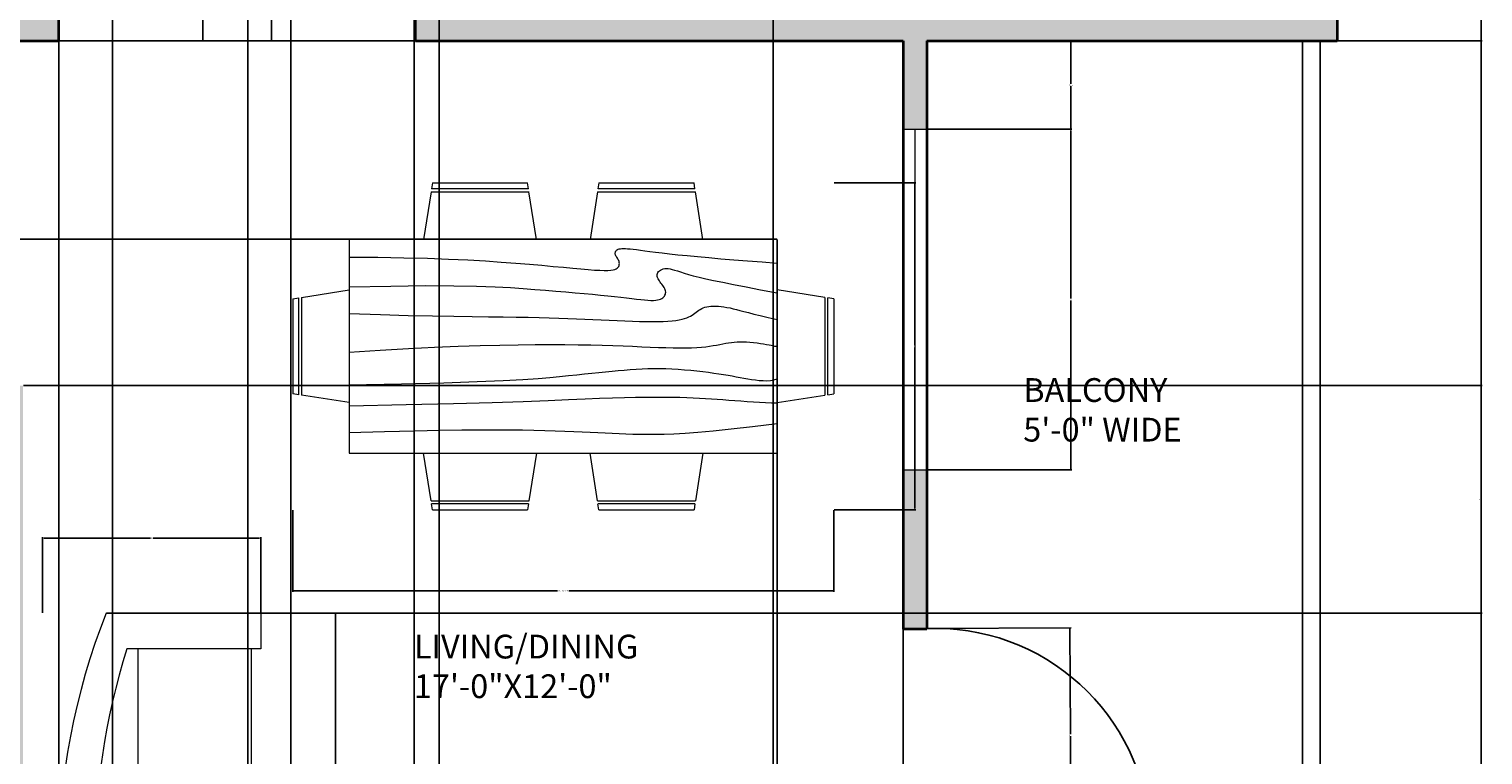
# Model space of a CAD drawing. Units: inches. Extents: x -29 to 443, y -589 to 39.
# Tile 4 of 5: x 139 to 384, y -275 to -153. Entities that reach past the tile are written whole.
import ezdxf

# ---------------------------------------------------------------- set-up
doc = ezdxf.new("R2010")
doc.units = ezdxf.units.IN
for name, color, linetype, lineweight in [('A-ANNO-DIMS', 2, 'Continuous', 18), ('A-AREA-IDEN', 7, 'Continuous', 18), ('A-DOOR', 3, 'Continuous', 25), ('A-FLOR-HRAL', 8, 'Continuous', 25), ('A-FURN', 9, 'Continuous', 18), ('A-GLAZ', 4, 'Continuous', 18), ('A-WALL', 7, 'Continuous', 35)]:
    doc.layers.add(name, color=color, linetype=linetype, lineweight=lineweight)
doc.layers.add('A-WALL-PATT', color=251, linetype='Continuous', lineweight=13, true_color=0x636466)
doc.styles.get("Standard").update_dxf_attribs({"font": 'arial.ttf'})
doc.dimstyles.get("Standard").update_dxf_attribs({"dimtxt": 0.18, "dimasz": 0.18, "dimexe": 0.18, "dimexo": 0.0625, "dimgap": 0.09, "dimtad": 0, "dimtih": 1, "dimtoh": 1, "dimdec": 4, "dimzin": 0, "dimdsep": 46, "dimtxsty": 'Standard', "dimcen": 0.09, "dimadec": 0, "dimazin": 0, "dimtfac": 1, "dimtdec": 4, "dimtofl": 0, "dimtmove": 0, "dimatfit": 3, "dimfxl": 1, "dimtolj": 1, "dimtzin": 0, "dimarcsym": 0})

# ---------------------------------------------------------------- blocks, each defined once
blk = doc.blocks.new('*U3')
for p, q in [((0, 0), (0, -6)), ((40, 0), (40, -6))]:
    blk.add_line(p, q)
blk.add_lwpolyline([(0, 0), (0, 40), (1.75, 40), (1.75, 0)], close=True)
blk.add_arc((0, 0), 40, 0, 90)
blk = doc.blocks.new('Sofa - Roundback 7 ft.')
for p, q in [((-12.00002, -32.4421), (-12.00003, -6.5971)), ((11.99997, -32.4421), (11.99998, -6.5971)), ((-36.000027, -34), (-36.000027, -11.4696)), ((35.99998, -34), (35.99998, -11.4696)), ((-35.999844, -13.3819), (35.9998, -13.3819)), ((-36.000027, -32.4421), (35.99998, -32.4421))]:
    blk.add_line(p, q)
for points in [[(-36.000027, -34), (-42.000027, -34), (-42.000027, -8)], [(41.99998, -8), (41.99998, -34), (35.99998, -34)]]:
    blk.add_lwpolyline(points)
for centre, radius, start, end in [((0, -114.25), 114.25, 68.43141, 111.5686), ((-0.00001, -127.1968), 121.1968, 72.72033, 107.2797)]:
    blk.add_arc(centre, radius, start, end)
blk = doc.blocks.new('Dining Set - 36 x 72 in.')
for p, q in [((-22, 27.5), (-22.1562, 26.50042)), ((-22, 27.5), (-6, 27.5)), ((-5.8437, 26.49966), (-6, 27.5)), ((6, 27.5), (5.8438, 26.50042)), ((6, 27.5), (22, 27.5)), ((22.1563, 26.49966), (22, 27.5)), ((-22.2343, 26.00059), (-23.4847, 17.99762)), ((-22.2304, 26), (-5.7608, 26)), ((-5.8416, 26.5), (-22.1534, 26.5)), ((-4.5152, 17.99762), (-5.7655, 25.99926)), ((5.7657, 26.00059), (4.5153, 17.99762)), ((5.7696, 26), (22.2392, 26)), ((22.1584, 26.5), (5.8466, 26.5)), ((23.4848, 17.99762), (22.2345, 25.99926)), ((36, 18), (-36, 18)), ((-36, 18), (-36, -18)), ((36, -18), (36, 18)), ((-45.5, 8), (-44.5004, 8.15617)), ((-45.5, 8), (-45.5, -8)), ((-44.5, -8.15843), (-44.5, 8.15338)), ((-44.0006, 8.23428), (-35.9976, 9.48474)), ((-44, 8.23041), (-44, -8.23915)), ((44.0006, 8.23428), (35.9976, 9.48474)), ((44, 8.23041), (44, -8.23915)), ((44.5, -8.15843), (44.5, 8.15338)), ((45.5, 8), (44.5005, 8.15617)), ((45.5, 8), (45.5, -8)), ((-44.4997, -8.15631), (-45.5, -8)), ((-35.9976, -9.48476), (-43.9993, -8.2345)), ((35.9976, -9.48476), (43.9993, -8.2345)), ((44.4997, -8.15631), (45.5, -8)), ((-36, -18), (36, -18)), ((-22.2343, -26.0006), (-23.4847, -17.99762)), ((-4.5152, -17.99762), (-5.7655, -25.99928)), ((5.7657, -26.0006), (4.5153, -17.99762)), ((23.4848, -17.99762), (22.2345, -25.99928)), ((-22.2304, -26), (-5.7608, -26)), ((-22, -27.5), (-22.1562, -26.50044)), ((-5.8416, -26.5), (-22.1534, -26.5)), ((-5.8437, -26.49967), (-6, -27.5)), ((5.7696, -26), (22.2392, -26)), ((6, -27.5), (5.8438, -26.50044)), ((22.1584, -26.5), (5.8466, -26.5)), ((22.1563, -26.49967), (22, -27.5)), ((-22, -27.5), (-6, -27.5)), ((6, -27.5), (22, -27.5))]:
    blk.add_line(p, q)
for points in [[(-36, 15), (-31.1772, 14.97754), (-26.8079, 14.91406), (-22.8538, 14.81543), (-19.276, 14.6875), (-16.0362, 14.53613), (-13.0957, 14.36718), (-10.4159, 14.18652), (-7.9583, 14), (-5.6904, 13.81315), (-3.6035, 13.63021), (-1.6954, 13.45508), (0.0365, 13.29166), (1.5945, 13.14388), (2.9811, 13.01562), (4.1988, 12.9108), (5.25, 12.83333), (6.1393, 12.78613), (6.8802, 12.76823), (7.4883, 12.77767), (7.9792, 12.8125), (8.3685, 12.87077), (8.6719, 12.95052), (8.9049, 13.0498), (9.0833, 13.16666), (9.2205, 13.29899), (9.3216, 13.44401), (9.3895, 13.59879), (9.4271, 13.76041), (9.4373, 13.92594), (9.4232, 14.09245), (9.3875, 14.257), (9.3333, 14.41666), (9.2638, 14.56917), (9.1836, 14.71484), (9.0975, 14.85465), (9.0104, 14.98958), (8.9272, 15.1206), (8.8529, 15.2487), (8.7922, 15.37483), (8.75, 15.5), (8.7305, 15.62467), (8.7344, 15.74739), (8.7617, 15.86621), (8.8125, 15.97916), (8.8867, 16.08431), (8.9844, 16.17968), (9.1055, 16.26334), (9.25, 16.33333), (9.4189, 16.38802), (9.6172, 16.42708), (9.8506, 16.45052), (10.125, 16.45833), (10.4463, 16.45052), (10.8203, 16.42708), (11.2529, 16.38802), (11.75, 16.33333), (12.3184, 16.26318), (12.9694, 16.17838), (13.7151, 16.07991), (14.5677, 15.96875), (15.5395, 15.84586), (16.6426, 15.71224), (17.8893, 15.56884), (19.2917, 15.41666), (20.859, 15.25667), (22.5879, 15.08984), (24.4721, 14.91715), (26.5052, 14.73958), (28.6809, 14.5581), (30.9929, 14.3737), (33.4347, 14.18733), (36, 14)], [(-36, 10), (-28.9766, 10.14274), (-23.1725, 10.20442), (-18.4241, 10.19775), (-14.5677, 10.13541), (-11.4399, 10.03011), (-8.877, 9.89453), (-6.7154, 9.74137), (-4.7917, 9.58333), (-2.9698, 9.43082), (-1.2246, 9.28515), (0.4415, 9.14534), (2.026, 9.01041), (3.5266, 8.87939), (4.9408, 8.7513), (6.266, 8.62516), (7.5, 8.5), (8.6411, 8.37549), (9.6914, 8.2539), (10.6538, 8.13818), (11.5312, 8.03125), (12.3267, 7.93603), (13.043, 7.85547), (13.6831, 7.79248), (14.25, 7.75), (14.7471, 7.7303), (15.1797, 7.73307), (15.5537, 7.75732), (15.875, 7.80208), (16.1494, 7.86637), (16.3828, 7.94922), (16.5811, 8.04964), (16.75, 8.16666), (16.8944, 8.29915), (17.0143, 8.44531), (17.1089, 8.60319), (17.1771, 8.77083), (17.218, 8.94629), (17.2305, 9.1276), (17.2137, 9.31282), (17.1667, 9.5), (17.0895, 9.6875), (16.987, 9.875), (16.8649, 10.0625), (16.7292, 10.25), (16.5856, 10.4375), (16.4401, 10.625), (16.2985, 10.8125), (16.1667, 11), (16.05, 11.18733), (15.9518, 11.3737), (15.8752, 11.5581), (15.8229, 11.73958), (15.798, 11.91715), (15.8034, 12.08984), (15.842, 12.25667), (15.9167, 12.41666), (16.0295, 12.56836), (16.1784, 12.70833), (16.3605, 12.83268), (16.5729, 12.9375), (16.8127, 13.01888), (17.0768, 13.07291), (17.3625, 13.0957), (17.6667, 13.08333), (17.9894, 13.03312), (18.3418, 12.94726), (18.7382, 12.82918), (19.1927, 12.68229), (19.7195, 12.51001), (20.3327, 12.31575), (21.0465, 12.10294), (21.875, 11.875), (22.8357, 11.63354), (23.959, 11.37304), (25.2786, 11.08618), (26.8282, 10.76562), (28.6414, 10.40405), (30.752, 9.99414), (33.1936, 9.52856), (36, 9)], [(-36, 5.5), (-30.7157, 5.3348), (-26.069, 5.20963), (-21.9946, 5.11767), (-18.4271, 5.05208), (-15.3009, 5.00602), (-12.5508, 4.97265), (-10.1112, 4.94515), (-7.9167, 4.91666), (-5.909, 4.88167), (-4.0586, 4.83984), (-2.3429, 4.79215), (-0.7396, 4.73958), (0.7739, 4.6831), (2.22, 4.6237), (3.6213, 4.56233), (5, 4.5), (6.373, 4.43782), (7.7344, 4.3776), (9.0723, 4.32129), (10.375, 4.27083), (11.6309, 4.22819), (12.8281, 4.19531), (13.9551, 4.17415), (15, 4.16666), (15.954, 4.17448), (16.819, 4.19791), (17.6001, 4.23698), (18.3021, 4.29166), (18.9299, 4.36198), (19.4883, 4.44791), (19.9823, 4.54948), (20.4167, 4.66666), (20.7969, 4.79899), (21.1302, 4.94401), (21.4245, 5.09879), (21.6875, 5.26041), (21.9271, 5.42594), (22.1511, 5.59245), (22.3672, 5.757), (22.5834, 5.91666), (22.8065, 6.06868), (23.0404, 6.21093), (23.2879, 6.34147), (23.5521, 6.45833), (23.8358, 6.55957), (24.142, 6.64323), (24.4735, 6.70735), (24.8334, 6.75), (25.2235, 6.76969), (25.642, 6.76692), (26.0858, 6.74267), (26.5521, 6.69791), (27.0379, 6.63362), (27.5404, 6.55078), (28.0565, 6.45036), (28.5834, 6.33333), (29.1242, 6.19987), (29.7071, 6.04687), (30.3661, 5.87044), (31.1354, 5.66666), (32.0493, 5.43164), (33.142, 5.16146), (34.4475, 4.85221), (36, 4.5)], [(-36, -1), (-30.7915, -0.6591), (-26.0195, -0.38216), (-21.6519, -0.16284), (-17.6563, 0.00521), (-14.0005, 0.12833), (-10.6523, 0.21289), (-7.5796, 0.26522), (-4.75, 0.29166), (-2.134, 0.29793), (0.2878, 0.28711), (2.5317, 0.26163), (4.6146, 0.22396), (6.5529, 0.17651), (8.3633, 0.12174), (10.0623, 0.06209), (11.6667, 0), (13.1899, -0.06201), (14.6341, -0.1211), (15.9982, -0.17432), (17.2813, -0.21875), (18.4823, -0.25147), (19.6003, -0.26953), (20.6343, -0.27002), (21.5834, -0.25), (22.4481, -0.20768), (23.2357, -0.14584), (23.9549, -0.06836), (24.6146, 0.02083), (25.2235, 0.11784), (25.7904, 0.21875), (26.3241, 0.31966), (26.8334, 0.41666), (27.3265, 0.50618), (27.8099, 0.58593), (28.2894, 0.65397), (28.7709, 0.70833), (29.2601, 0.74707), (29.763, 0.76823), (30.2855, 0.76985), (30.8334, 0.75), (31.4088, 0.70784), (31.9994, 0.64713), (32.589, 0.57275), (33.1615, 0.48958), (33.7008, 0.4025), (34.1908, 0.3164), (34.6153, 0.23616), (34.9584, 0.16666), (35.2099, 0.11165), (35.3848, 0.07031), (35.504, 0.04069), (35.5886, 0.02083), (35.6594, 0.00879), (35.7377, 0.0026), (35.8442, 0.00032), (36, 0)], [(-36, -6.5), (-27.1843, -6.31267), (-20.084, -6.1263), (-14.469, -5.9419), (-10.1094, -5.76042), (-6.7752, -5.58285), (-4.2363, -5.41016), (-2.2629, -5.24333), (-0.625, -5.08334), (0.8708, -4.93099), (2.2715, -4.78646), (3.5872, -4.64974), (4.8281, -4.52084), (6.0046, -4.39974), (7.127, -4.28646), (8.2053, -4.18099), (9.25, -4.08334), (10.2705, -3.99382), (11.2734, -3.91407), (12.2647, -3.84603), (13.25, -3.79167), (14.2354, -3.75293), (15.2266, -3.73177), (16.2295, -3.73015), (17.25, -3.75), (18.2912, -3.79248), (19.3451, -3.85547), (20.4009, -3.93604), (21.4479, -4.03125), (22.4754, -4.13819), (23.4727, -4.25391), (24.4289, -4.37549), (25.3334, -4.5), (26.1785, -4.62492), (26.9694, -4.74935), (27.7145, -4.87281), (28.4219, -4.99479), (29.1, -5.11483), (29.7572, -5.23242), (30.4016, -5.34709), (31.0417, -5.45834), (31.6837, -5.56437), (32.3262, -5.65821), (32.9658, -5.73153), (33.599, -5.77604), (34.2224, -5.78345), (34.8327, -5.74545), (35.4264, -5.65373), (36, -5.5)], [(-36, -10), (-26.4022, -9.81299), (-18.4675, -9.62891), (-11.9839, -9.45069), (-6.7396, -9.28125), (-2.5226, -9.12354), (0.8789, -8.98047), (3.6769, -8.85498), (6.0833, -8.75), (8.2767, -8.66765), (10.3021, -8.60677), (12.1712, -8.56543), (13.8958, -8.54167), (15.4876, -8.53353), (16.9583, -8.53907), (18.3197, -8.55632), (19.5834, -8.58334), (20.7616, -8.61841), (21.8685, -8.66081), (22.9188, -8.71004), (23.9271, -8.76563), (24.9081, -8.82707), (25.8763, -8.89388), (26.8465, -8.96558), (27.8334, -9.04167), (28.8474, -9.12118), (29.8828, -9.20117), (30.93, -9.27824), (31.9792, -9.34896), (33.0205, -9.40991), (34.0443, -9.45768), (35.0407, -9.48885), (36, -9.5)], [(-36, -14.5), (-30.0881, -14.33513), (-25.0332, -14.21224), (-20.7312, -14.12647), (-17.0781, -14.07292), (-13.97, -14.04671), (-11.3027, -14.04297), (-8.9724, -14.05681), (-6.875, -14.08334), (-4.9224, -14.11833), (-3.0905, -14.16016), (-1.3709, -14.20785), (0.2448, -14.26042), (1.7647, -14.3169), (3.1973, -14.3763), (4.5507, -14.43767), (5.8333, -14.5), (7.0554, -14.5621), (8.235, -14.62175), (9.3922, -14.67652), (10.5469, -14.72396), (11.7192, -14.76164), (12.929, -14.78711), (14.1965, -14.79794), (15.5417, -14.79167), (16.9933, -14.76424), (18.6152, -14.70508), (20.4804, -14.60197), (22.6615, -14.44271), (25.2312, -14.21509), (28.2624, -13.9069), (31.8277, -13.50594), (36, -13)]]:
    blk.add_lwpolyline(points)
blk = doc.blocks.new('*D30')
at = {"layer": 'A-ANNO-DIMS', "color": 0, "lineweight": -2, "transparency": 16777216}
for p, q in [((178.45, -250.92), (191.17, -250.92)), ((190.99, -251.1), (190.99, -292.74)), ((190.99, -334.74), (190.99, -293.11)), ((178.45, -334.92), (191.17, -334.92))]:
    blk.add_line(p, q, dxfattribs=at)
at = {"layer": 'A-ANNO-DIMS', "color": 0, "transparency": 16777216}
for points in [[(190.96, -251.1), (191.02, -251.1), (190.99, -250.92)], [(190.96, -334.74), (191.02, -334.74), (190.99, -334.92)]]:
    blk.add_solid(points, dxfattribs=at)
at = {"layer": 'Defpoints', "color": 0, "transparency": 16777216}
for p in [(178.39, -250.92), (190.99, -250.92), (178.39, -334.92)]:
    blk.add_point(p, dxfattribs=at)
at = {"layer": 'A-ANNO-DIMS', "color": 0, "transparency": 16777216, "insert": (190.99, -292.92), "char_height": 0.18, "attachment_point": 5}
blk.add_mtext('\\A1;SOFA 84', dxfattribs=at)
blk = doc.blocks.new('*D31')
at = {"layer": 'A-ANNO-DIMS', "color": 0, "lineweight": -2, "transparency": 16777216}
for p, q in [((141.72, -250.86), (141.72, -238.14)), ((141.9, -238.32), (159.84, -238.32)), ((178.21, -238.32), (160.28, -238.32)), ((178.39, -250.86), (178.39, -238.14))]:
    blk.add_line(p, q, dxfattribs=at)
at = {"layer": 'A-ANNO-DIMS', "color": 0, "transparency": 16777216}
for points in [[(141.9, -238.29), (141.9, -238.35), (141.72, -238.32)], [(178.21, -238.29), (178.21, -238.35), (178.39, -238.32)]]:
    blk.add_solid(points, dxfattribs=at)
at = {"layer": 'Defpoints', "color": 0, "transparency": 16777216}
for p in [(141.72, -238.32), (141.72, -250.92), (178.39, -250.92)]:
    blk.add_point(p, dxfattribs=at)
at = {"layer": 'A-ANNO-DIMS', "color": 0, "transparency": 16777216, "insert": (160.06, -238.32), "char_height": 0.18, "attachment_point": 5}
blk.add_mtext('\\A1;37', dxfattribs=at)
blk = doc.blocks.new('*D32')
at = {"layer": 'A-ANNO-DIMS', "color": 0, "lineweight": -2, "transparency": 16777216}
for p, q in [((183.78, -233.57), (183.78, -247.33)), ((274.78, -233.57), (274.78, -247.33)), ((183.96, -247.15), (228.33, -247.15)), ((274.6, -247.15), (230.24, -247.15))]:
    blk.add_line(p, q, dxfattribs=at)
at = {"layer": 'A-ANNO-DIMS', "color": 0, "transparency": 16777216}
for points in [[(183.96, -247.12), (183.96, -247.18), (183.78, -247.15)], [(274.6, -247.12), (274.6, -247.18), (274.78, -247.15)]]:
    blk.add_solid(points, dxfattribs=at)
at = {"layer": 'Defpoints', "color": 0, "transparency": 16777216}
for p in [(183.78, -233.5), (274.78, -233.5), (274.78, -247.15)]:
    blk.add_point(p, dxfattribs=at)
at = {"layer": 'A-ANNO-DIMS', "color": 0, "transparency": 16777216, "insert": (229.28, -247.15), "char_height": 0.18, "attachment_point": 5}
blk.add_mtext('\\A1;DINING SET 91', dxfattribs=at)
blk = doc.blocks.new('*D33')
at = {"layer": 'A-ANNO-DIMS', "color": 0, "lineweight": -2, "transparency": 16777216}
for p, q in [((274.85, -178.5), (288.61, -178.5)), ((288.43, -178.68), (288.43, -205.82)), ((288.43, -233.32), (288.43, -206.18)), ((274.85, -233.5), (288.61, -233.5))]:
    blk.add_line(p, q, dxfattribs=at)
at = {"layer": 'A-ANNO-DIMS', "color": 0, "transparency": 16777216}
for points in [[(288.4, -178.68), (288.46, -178.68), (288.43, -178.5)], [(288.4, -233.32), (288.46, -233.32), (288.43, -233.5)]]:
    blk.add_solid(points, dxfattribs=at)
at = {"layer": 'Defpoints', "color": 0, "transparency": 16777216}
for p in [(274.78, -178.5), (288.43, -178.5), (274.78, -233.5)]:
    blk.add_point(p, dxfattribs=at)
at = {"layer": 'A-ANNO-DIMS', "color": 0, "transparency": 16777216, "insert": (288.43, -206), "char_height": 0.18, "attachment_point": 5}
blk.add_mtext('\\A1;55', dxfattribs=at)
blk = doc.blocks.new('*D40')
at = {"layer": 'A-ANNO-DIMS', "color": 0, "lineweight": -2, "transparency": 16777216}
for p, q in [((208.44, 5.32), (208.44, -492.89)), ((264.58, 5.32), (264.58, -492.89)), ((208.62, -492.71), (236.11, -492.71)), ((264.4, -492.71), (236.9, -492.71))]:
    blk.add_line(p, q, dxfattribs=at)
at = {"layer": 'A-ANNO-DIMS', "color": 0, "transparency": 16777216}
for points in [[(208.62, -492.68), (208.62, -492.74), (208.44, -492.71)], [(264.4, -492.68), (264.4, -492.74), (264.58, -492.71)]]:
    blk.add_solid(points, dxfattribs=at)
at = {"layer": 'Defpoints', "color": 0, "transparency": 16777216}
for p in [(208.44, 5.39), (264.58, 5.39), (208.44, -492.71)]:
    blk.add_point(p, dxfattribs=at)
at = {"layer": 'A-ANNO-DIMS', "color": 0, "transparency": 16777216, "insert": (236.51, -492.71), "char_height": 0.18, "attachment_point": 5}
blk.add_mtext('\\A1;56.14', dxfattribs=at)
blk = doc.blocks.new('*D44')
at = {"layer": 'A-ANNO-DIMS', "color": 0, "lineweight": -2, "transparency": 16777216}
for p, q in [((359.5, 14.39), (383.85, 14.39)), ((383.67, 14.21), (383.67, -69.93)), ((383.67, -154.43), (383.67, -70.3)), ((359.5, -154.61), (383.85, -154.61))]:
    blk.add_line(p, q, dxfattribs=at)
at = {"layer": 'A-ANNO-DIMS', "color": 0, "transparency": 16777216}
for points in [[(383.64, 14.21), (383.7, 14.21), (383.67, 14.39)], [(383.64, -154.43), (383.7, -154.43), (383.67, -154.61)]]:
    blk.add_solid(points, dxfattribs=at)
at = {"layer": 'Defpoints', "color": 0, "transparency": 16777216}
for p in [(359.44, 14.39), (359.44, -154.61), (383.67, -154.61)]:
    blk.add_point(p, dxfattribs=at)
at = {"layer": 'A-ANNO-DIMS', "color": 0, "transparency": 16777216, "insert": (383.67, -70.11), "char_height": 0.18, "attachment_point": 5}
blk.add_mtext('\\A1;169', dxfattribs=at)
blk = doc.blocks.new('*D45')
at = {"layer": 'A-ANNO-DIMS', "color": 0, "lineweight": -2, "transparency": 16777216}
for p, q in [((359.5, -154.61), (383.85, -154.61)), ((383.67, -154.79), (383.67, -226.43)), ((383.67, -298.43), (383.67, -226.8)), ((359.5, -298.61), (383.85, -298.61))]:
    blk.add_line(p, q, dxfattribs=at)
at = {"layer": 'A-ANNO-DIMS', "color": 0, "transparency": 16777216}
for points in [[(383.64, -154.79), (383.7, -154.79), (383.67, -154.61)], [(383.64, -298.43), (383.7, -298.43), (383.67, -298.61)]]:
    blk.add_solid(points, dxfattribs=at)
at = {"layer": 'Defpoints', "color": 0, "transparency": 16777216}
for p in [(359.44, -154.61), (359.44, -298.61), (383.67, -298.61)]:
    blk.add_point(p, dxfattribs=at)
at = {"layer": 'A-ANNO-DIMS', "color": 0, "transparency": 16777216, "insert": (383.67, -226.61), "char_height": 0.18, "attachment_point": 5}
blk.add_mtext('\\A1;144', dxfattribs=at)
blk = doc.blocks.new('*D51')
at = {"layer": 'A-ANNO-DIMS', "color": 0, "lineweight": -2, "transparency": 16777216}
for p, q in [((144.5, -141.61), (168.85, -141.61)), ((168.67, -141.79), (168.67, -147.93)), ((168.67, -154.43), (168.67, -148.3)), ((144.5, -154.61), (168.85, -154.61))]:
    blk.add_line(p, q, dxfattribs=at)
at = {"layer": 'A-ANNO-DIMS', "color": 0, "transparency": 16777216}
for points in [[(168.64, -141.79), (168.7, -141.79), (168.67, -141.61)], [(168.64, -154.43), (168.7, -154.43), (168.67, -154.61)]]:
    blk.add_solid(points, dxfattribs=at)
at = {"layer": 'Defpoints', "color": 0, "transparency": 16777216}
for p in [(144.44, -141.61), (144.44, -154.61), (168.67, -154.61)]:
    blk.add_point(p, dxfattribs=at)
at = {"layer": 'A-ANNO-DIMS', "color": 0, "transparency": 16777216, "insert": (168.67, -148.11), "char_height": 0.18, "attachment_point": 5}
blk.add_mtext('\\A1;13', dxfattribs=at)
blk = doc.blocks.new('*D52')
at = {"layer": 'A-ANNO-DIMS', "color": 0, "lineweight": -2, "transparency": 16777216}
for p, q in [((153.44, -94.68), (153.44, -492.89)), ((183.44, -94.68), (183.44, -492.89)), ((153.62, -492.71), (168.22, -492.71)), ((183.26, -492.71), (168.65, -492.71))]:
    blk.add_line(p, q, dxfattribs=at)
at = {"layer": 'A-ANNO-DIMS', "color": 0, "transparency": 16777216}
for points in [[(153.62, -492.68), (153.62, -492.74), (153.44, -492.71)], [(183.26, -492.68), (183.26, -492.74), (183.44, -492.71)]]:
    blk.add_solid(points, dxfattribs=at)
at = {"layer": 'Defpoints', "color": 0, "transparency": 16777216}
for p in [(153.44, -94.61), (183.44, -94.61), (183.44, -492.71)]:
    blk.add_point(p, dxfattribs=at)
at = {"layer": 'A-ANNO-DIMS', "color": 0, "transparency": 16777216, "insert": (168.44, -492.71), "char_height": 0.18, "attachment_point": 5}
blk.add_mtext('\\A1;30', dxfattribs=at)
blk = doc.blocks.new('*D55')
at = {"layer": 'A-ANNO-DIMS', "color": 0, "lineweight": -2, "transparency": 16777216}
for p, q in [((290.34, -253.47), (314.69, -253.36)), ((314.51, -253.54), (314.59, -271.25)), ((314.66, -289.33), (314.59, -271.62)), ((290.5, -289.61), (314.85, -289.51))]:
    blk.add_line(p, q, dxfattribs=at)
at = {"layer": 'A-ANNO-DIMS', "color": 0, "transparency": 16777216}
for points in [[(314.54, -253.54), (314.48, -253.54), (314.51, -253.36)], [(314.69, -289.33), (314.63, -289.33), (314.67, -289.51)]]:
    blk.add_solid(points, dxfattribs=at)
at = {"layer": 'Defpoints', "color": 0, "transparency": 16777216}
for p in [(290.28, -253.47), (290.44, -289.61), (314.67, -289.51)]:
    blk.add_point(p, dxfattribs=at)
at = {"layer": 'A-ANNO-DIMS', "color": 0, "transparency": 16777216, "insert": (314.59, -271.44), "char_height": 0.18, "attachment_point": 5}
blk.add_mtext('\\A1;36.15', dxfattribs=at)
blk = doc.blocks.new('*D63')
at = {"layer": 'A-ANNO-DIMS', "color": 0, "lineweight": -2, "transparency": 16777216}
for p, q in [((204.37, -144.61), (180.03, -144.61)), ((180.21, -144.79), (180.21, -149.43)), ((180.21, -154.43), (180.21, -149.8)), ((204.37, -154.61), (180.03, -154.61))]:
    blk.add_line(p, q, dxfattribs=at)
at = {"layer": 'A-ANNO-DIMS', "color": 0, "transparency": 16777216}
for points in [[(180.18, -144.79), (180.24, -144.79), (180.21, -144.61)], [(180.18, -154.43), (180.24, -154.43), (180.21, -154.61)]]:
    blk.add_solid(points, dxfattribs=at)
at = {"layer": 'Defpoints', "color": 0, "transparency": 16777216}
for p in [(180.21, -144.61), (204.44, -144.61), (204.44, -154.61)]:
    blk.add_point(p, dxfattribs=at)
at = {"layer": 'A-ANNO-DIMS', "color": 0, "transparency": 16777216, "insert": (180.21, -149.61), "char_height": 0.18, "attachment_point": 5}
blk.add_mtext('\\A1;10', dxfattribs=at)
blk = doc.blocks.new('*D68')
at = {"layer": 'A-ANNO-DIMS', "color": 0, "lineweight": -2, "transparency": 16777216}
for p, q in [((176.21, -22.71), (176.21, -492.89)), ((204.21, -33.21), (204.21, -492.89)), ((176.39, -492.71), (189.99, -492.71)), ((204.03, -492.71), (190.43, -492.71))]:
    blk.add_line(p, q, dxfattribs=at)
at = {"layer": 'A-ANNO-DIMS', "color": 0, "transparency": 16777216}
for points in [[(176.39, -492.68), (176.39, -492.74), (176.21, -492.71)], [(204.03, -492.68), (204.03, -492.74), (204.21, -492.71)]]:
    blk.add_solid(points, dxfattribs=at)
at = {"layer": 'Defpoints', "color": 0, "transparency": 16777216}
for p in [(176.21, -22.65), (204.21, -33.15), (204.21, -492.71)]:
    blk.add_point(p, dxfattribs=at)
at = {"layer": 'A-ANNO-DIMS', "color": 0, "transparency": 16777216, "insert": (190.21, -492.71), "char_height": 0.18, "attachment_point": 5}
blk.add_mtext('\\A1;28', dxfattribs=at)
blk = doc.blocks.new('*D71')
at = {"layer": 'A-ANNO-DIMS', "color": 0, "lineweight": -2, "transparency": 16777216}
for p, q in [((144.44, -94.68), (144.44, -492.89)), ((153.44, -94.68), (153.44, -492.89)), ((144.62, -492.71), (148.79, -492.71)), ((153.26, -492.71), (149.09, -492.71))]:
    blk.add_line(p, q, dxfattribs=at)
at = {"layer": 'A-ANNO-DIMS', "color": 0, "transparency": 16777216}
for points in [[(144.62, -492.68), (144.62, -492.74), (144.44, -492.71)], [(153.26, -492.68), (153.26, -492.74), (153.44, -492.71)]]:
    blk.add_solid(points, dxfattribs=at)
at = {"layer": 'Defpoints', "color": 0, "transparency": 16777216}
for p in [(144.44, -94.61), (153.44, -94.61), (153.44, -492.71)]:
    blk.add_point(p, dxfattribs=at)
at = {"layer": 'A-ANNO-DIMS', "color": 0, "transparency": 16777216, "insert": (148.94, -492.71), "char_height": 0.18, "attachment_point": 5}
blk.add_mtext('\\A1;9', dxfattribs=at)
blk = doc.blocks.new('*D74')
at = {"layer": 'A-ANNO-DIMS', "color": 0, "lineweight": -2, "transparency": 16777216}
for p, q in [((286.44, -169.54), (286.44, -492.89)), ((265.28, -188.07), (265.28, -492.89)), ((265.46, -492.71), (275.46, -492.71)), ((286.26, -492.71), (276.26, -492.71))]:
    blk.add_line(p, q, dxfattribs=at)
at = {"layer": 'A-ANNO-DIMS', "color": 0, "transparency": 16777216}
for points in [[(265.46, -492.68), (265.46, -492.74), (265.28, -492.71)], [(286.26, -492.68), (286.26, -492.74), (286.44, -492.71)]]:
    blk.add_solid(points, dxfattribs=at)
at = {"layer": 'Defpoints', "color": 0, "transparency": 16777216}
for p in [(286.44, -169.48), (265.28, -188), (286.44, -492.71)]:
    blk.add_point(p, dxfattribs=at)
at = {"layer": 'A-ANNO-DIMS', "color": 0, "transparency": 16777216, "insert": (275.86, -492.71), "char_height": 0.18, "attachment_point": 5}
blk.add_mtext('\\A1;21.15', dxfattribs=at)
blk = doc.blocks.new('*D75')
at = {"layer": 'A-ANNO-DIMS', "color": 0, "lineweight": -2, "transparency": 16777216}
for p, q in [((286.37, -154.61), (-28.85, -154.61)), ((-28.67, -154.79), (-28.67, -171.13)), ((-28.67, -187.82), (-28.67, -171.49)), ((265.22, -188), (-28.85, -188))]:
    blk.add_line(p, q, dxfattribs=at)
at = {"layer": 'A-ANNO-DIMS', "color": 0, "transparency": 16777216}
for points in [[(-28.7, -154.79), (-28.64, -154.79), (-28.67, -154.61)], [(-28.7, -187.82), (-28.64, -187.82), (-28.67, -188)]]:
    blk.add_solid(points, dxfattribs=at)
at = {"layer": 'Defpoints', "color": 0, "transparency": 16777216}
for p in [(-28.67, -154.61), (286.44, -154.61), (265.28, -188)]:
    blk.add_point(p, dxfattribs=at)
at = {"layer": 'A-ANNO-DIMS', "color": 0, "transparency": 16777216, "insert": (-28.67, -171.31), "char_height": 0.18, "attachment_point": 5}
blk.add_mtext('\\A1;33.39', dxfattribs=at)
blk = doc.blocks.new('*D77')
at = {"layer": 'A-ANNO-DIMS', "color": 0, "lineweight": -2, "transparency": 16777216}
for p, q in [((290.5, -154.61), (314.85, -154.61)), ((314.67, -154.79), (314.67, -161.86)), ((314.67, -169.3), (314.67, -162.23)), ((290.5, -169.48), (314.85, -169.48))]:
    blk.add_line(p, q, dxfattribs=at)
at = {"layer": 'A-ANNO-DIMS', "color": 0, "transparency": 16777216}
for points in [[(314.64, -154.79), (314.7, -154.79), (314.67, -154.61)], [(314.64, -169.3), (314.7, -169.3), (314.67, -169.48)]]:
    blk.add_solid(points, dxfattribs=at)
at = {"layer": 'Defpoints', "color": 0, "transparency": 16777216}
for p in [(290.44, -154.61), (290.44, -169.48), (314.67, -169.48)]:
    blk.add_point(p, dxfattribs=at)
at = {"layer": 'A-ANNO-DIMS', "color": 0, "transparency": 16777216, "insert": (314.67, -162.05), "char_height": 0.18, "attachment_point": 5}
blk.add_mtext('\\A1;14.863', dxfattribs=at)
blk = doc.blocks.new('*D78')
at = {"layer": 'A-ANNO-DIMS', "color": 0, "lineweight": -2, "transparency": 16777216}
for p, q in [((290.5, -169.48), (314.85, -169.48)), ((314.67, -169.66), (314.67, -197.95)), ((314.67, -226.61), (314.67, -198.32)), ((290.5, -226.79), (314.85, -226.79))]:
    blk.add_line(p, q, dxfattribs=at)
at = {"layer": 'A-ANNO-DIMS', "color": 0, "transparency": 16777216}
for points in [[(314.64, -169.66), (314.7, -169.66), (314.67, -169.48)], [(314.64, -226.61), (314.7, -226.61), (314.67, -226.79)]]:
    blk.add_solid(points, dxfattribs=at)
at = {"layer": 'Defpoints', "color": 0, "transparency": 16777216}
for p in [(290.44, -169.48), (290.44, -226.79), (314.67, -226.79)]:
    blk.add_point(p, dxfattribs=at)
at = {"layer": 'A-ANNO-DIMS', "color": 0, "transparency": 16777216, "insert": (314.67, -198.13), "char_height": 0.18, "attachment_point": 5}
blk.add_mtext('\\A1;57.31', dxfattribs=at)
blk = doc.blocks.new('*D82')
at = {"layer": 'A-ANNO-DIMS', "color": 0, "lineweight": -2, "transparency": 16777216}
for p, q in [((138.5, -212.61), (383.85, -212.61)), ((383.67, -212.79), (383.67, -231.59)), ((383.67, -250.74), (383.67, -231.95)), ((152.45, -250.92), (383.85, -250.92))]:
    blk.add_line(p, q, dxfattribs=at)
at = {"layer": 'A-ANNO-DIMS', "color": 0, "transparency": 16777216}
for points in [[(383.64, -212.79), (383.7, -212.79), (383.67, -212.61)], [(383.64, -250.74), (383.7, -250.74), (383.67, -250.92)]]:
    blk.add_solid(points, dxfattribs=at)
at = {"layer": 'Defpoints', "color": 0, "transparency": 16777216}
for p in [(138.44, -212.61), (152.39, -250.92), (383.67, -250.92)]:
    blk.add_point(p, dxfattribs=at)
at = {"layer": 'A-ANNO-DIMS', "color": 0, "transparency": 16777216, "insert": (383.67, -231.77), "char_height": 0.18, "attachment_point": 5}
blk.add_mtext('\\A1;38.31', dxfattribs=at)

msp = doc.modelspace()

# ---------------------------------------------------------------- hatches: boundary and pattern name
at = {"layer": 'A-WALL-PATT'}
h = msp.add_hatch(color=256, dxfattribs=at)
h.dxf.hatch_style = 1
h.paths.add_polyline_path([(8.4359, 5.3851), (38.6638, 5.3851), (38.6638, 14.3851), (-0.5641, 14.3851), (-0.5641, -161.7206), (8.4359, -161.7206), (8.4359, -154.6149), (98.4359, -154.6149), (98.4359, -169.6149), (102.4359, -169.6149), (102.4359, -154.6149), (144.4359, -154.6149), (144.4359, -141.6149), (140.4359, -141.6149), (140.4359, -150.6149), (8.4359, -150.6149)])
h.paths.add_polyline_path([(153.762, 14.3851), (92.6638, 14.3851), (92.6638, 5.3851), (140.4359, 5.3851), (140.4359, -105.5868), (144.4359, -105.5868), (144.4359, -94.6149), (153.4359, -94.6149), (153.4359, -90.6149), (144.4359, -90.6149), (144.4359, 5.3851), (153.762, 5.3851)])
h.paths.add_polyline_path([(264.576, 14.3851), (189.762, 14.3851), (189.762, 5.3851), (204.4359, 5.3851), (204.4359, -40.0486, -0.11439146), (204.5889, -40.7086), (204.5889, -67.7086, -0.11439146), (204.4359, -68.3685), (204.4359, -90.6149), (183.4359, -90.6149), (183.4359, -94.6149), (204.4359, -94.6149), (204.4359, -108.4622), (208.4359, -108.4622), (208.4359, 5.3851), (264.576, 5.3851)])
h.paths.add_polyline_path([(359.4359, 14.3851), (318.576, 14.3851), (318.576, 5.3851), (350.4359, 5.3851), (350.4359, -150.6149), (208.4359, -150.6149), (208.4359, -144.6149), (204.4359, -144.6149), (204.4359, -154.6149), (286.4359, -154.6149), (286.4359, -169.4775), (290.4359, -169.4775), (290.4359, -154.6149), (359.4359, -154.6149)])
h.paths.add_polyline_path([(8.4359, -212.6149), (98.4359, -212.6149), (102.4359, -212.6149), (102.4359, -199.6149), (98.4359, -199.6149), (98.4359, -208.6149), (8.4359, -208.6149), (8.4359, -197.7206), (-0.5641, -197.7206), (-0.5641, -417.6149), (114.4359, -417.6149), (114.4359, -354.6149), (134.4359, -354.6149), (134.4359, -453.6149), (147.4359, -453.6149), (147.4359, -444.6149), (138.4359, -444.6149), (138.4359, -212.6149), (129.4359, -212.6149), (129.4359, -216.6149), (134.4359, -216.6149), (134.4359, -350.6149), (110.4359, -350.6149), (110.4359, -377.2063, -0.30395766), (111.1497, -378.2719, -0.30395766), (110.4359, -379.3376), (110.4359, -408.6149), (8.4359, -408.6149)])
h.paths.add_polyline_path([(265.0252, -444.6149), (230.4359, -444.6149), (230.4359, -396.6149), (246.223, -396.6149), (246.223, -392.6149), (230.4359, -392.6149), (230.4359, -302.6149), (245.4886, -302.6149), (245.4886, -298.6149), (226.4359, -298.6149), (226.4359, -444.6149), (189.4359, -444.6149), (189.4359, -453.6149), (226.4359, -453.6149), (265.0252, -453.6149)])
h.paths.add_polyline_path([(359.4359, -417.6149), (359.4359, -377.3771), (350.4359, -377.3771), (350.4359, -392.6149), (276.3235, -392.6149), (276.3235, -396.6149), (350.4359, -396.6149), (350.4359, -408.6149), (350.4359, -444.6149), (319.0252, -444.6149), (319.0252, -453.6149), (359.4359, -453.6149)])
h.paths.add_polyline_path([(359.4359, -298.6149), (290.4359, -298.6149), (290.4359, -289.6207), (286.4359, -289.6207), (286.4359, -298.6149), (277.8355, -298.6149), (277.8355, -302.6149), (350.4359, -302.6149), (350.4359, -323.3771), (359.4359, -323.3771)])
h.paths.add_polyline_path([(290.4359, -226.7916), (286.4359, -226.7916), (286.4359, -253.468), (290.4359, -253.468)])

# ---------------------------------------------------------------- linework, layer by layer
at = {"layer": 'A-FLOR-HRAL'}
for p, q in [((353.5994, -154.6149), (353.5994, -298.6149)), ((356.5994, -154.6149), (356.5994, -298.6149))]:
    msp.add_line(p, q, dxfattribs=at)
at = {"layer": 'A-GLAZ'}
for p, q in [((286.4359, -169.4775), (290.4359, -169.4775)), ((288.4359, -169.4775), (288.4359, -226.7916)), ((286.4359, -226.7916), (290.4359, -226.7916))]:
    msp.add_line(p, q, dxfattribs=at)
at = {"layer": 'A-WALL'}
for p, q in [((359.4359, 14.3851), (359.4359, -154.6149)), ((144.4359, -154.6149), (144.4359, -141.6149)), ((204.4359, -154.6149), (204.4359, -144.6149)), ((102.4359, -154.6149), (144.4359, -154.6149)), ((204.4359, -154.6149), (286.4359, -154.6149)), ((286.4359, -154.6149), (286.4359, -253.6149)), ((290.4359, -154.6149), (290.4359, -253.6149)), ((290.4359, -154.6149), (359.4359, -154.6149)), ((290.4359, -253.6149), (286.4359, -253.6149))]:
    msp.add_line(p, q, dxfattribs=at)

# ---------------------------------------------------------------- block references
at = {"layer": 'A-DOOR', "xscale": -0.9038178546105021, "yscale": 0.9038178546105021, "zscale": 0.9038178546105021, "rotation": 270}
msp.add_blockref('*U3', (291.8589, -289.6207), dxfattribs=at)
at = {"layer": 'A-FURN'}
msp.add_blockref('Dining Set - 36 x 72 in.', (229.284, -206.0033), dxfattribs=at)
at = {"layer": 'A-FURN', "rotation": 89.99999967709844}
msp.add_blockref('Sofa - Roundback 7 ft.', (144.3905, -292.9234), dxfattribs=at)

# ---------------------------------------------------------------- texts
at = {"layer": 'A-AREA-IDEN', "char_height": 4, "attachment_point": 1}
for s, width, insert in [('BALCONY\\P5\'-0" WIDE', 32.234328, (306.6588, -211.3646)), ('LIVING/DINING\\P17\'-0"X12\'-0"', 54.511225, (204.1648, -254.5404))]:
    msp.add_mtext_dynamic_manual_height_columns(s, width=width, gutter_width=12.5, heights=[0], dxfattribs=dict(at, insert=insert))

# ---------------------------------------------------------------- dimensions: what is measured, and where the dimension line sits
at = {"layer": 'A-ANNO-DIMS'}
for base, p1, p2, angle, override, picture, middle in [((383.6659, -154.6149), (359.4359, 14.3851), (359.4359, -154.6149), 90, {"dimdec": 0, "dimlfac": 1, "dimrnd": 0, "dimzin": 0, "dimdsep": 46, "dimlunit": 2}, '*D44', (383.6659, -70.1149)), ((168.6659, -154.6149), (144.4359, -141.6149), (144.4359, -154.6149), 270, {"dimdec": 0, "dimlfac": 1, "dimrnd": 0, "dimzin": 0, "dimdsep": 46, "dimlunit": 2}, '*D51', (168.6659, -148.1149)), ((180.2059, -144.6149), (204.4359, -154.6149), (204.4359, -144.6149), 90, {"dimdec": 0, "dimlfac": 1, "dimrnd": 0, "dimzin": 0, "dimdsep": 46, "dimlunit": 2}, '*D63', (180.2059, -149.6149)), ((-28.6698, -154.6149), (265.284, -188.0033), (286.4359, -154.6149), 90, {"dimdec": 2, "dimlfac": 1, "dimrnd": 0, "dimzin": 0, "dimdsep": 46, "dimlunit": 2}, '*D75', (-28.6698, -171.3091)), ((314.6659, -169.4775), (290.4359, -154.6149), (290.4359, -169.4775), 270, {"dimdec": 3, "dimlfac": 1, "dimrnd": 0, "dimzin": 0, "dimdsep": 46, "dimlunit": 2}, '*D77', (314.6659, -162.0462)), ((383.6659, -298.6149), (359.4359, -154.6149), (359.4359, -298.6149), 90, {"dimdec": 0, "dimlfac": 1, "dimrnd": 0, "dimzin": 0, "dimdsep": 46, "dimlunit": 2}, '*D45', (383.6659, -226.6149)), ((314.6659, -226.7916), (290.4359, -169.4775), (290.4359, -226.7916), 270, {"dimdec": 2, "dimlfac": 1, "dimrnd": 0, "dimzin": 0, "dimdsep": 46, "dimlunit": 2}, '*D78', (314.6659, -198.1345)), ((288.434, -178.5033), (274.784, -233.5033), (274.784, -178.5033), 90, {"dimdec": 0, "dimlfac": 1, "dimrnd": 0, "dimzin": 0, "dimdsep": 46, "dimlunit": 2}, '*D33', (288.434, -206.0033)), ((383.6659, -250.9234), (138.4359, -212.6149), (152.3905, -250.9234), 90, {"dimdec": 2, "dimlfac": 1, "dimrnd": 0, "dimzin": 0, "dimdsep": 46, "dimlunit": 2}, '*D82', (383.6659, -231.7692)), ((141.7238, -238.3234), (178.3905, -250.9234), (141.7238, -250.9234), 180, {"dimdec": 0, "dimlfac": 1, "dimrnd": 0, "dimzin": 0, "dimdsep": 46, "dimlunit": 2}, '*D31', (160.0572, -238.3234)), ((314.6657, -289.5085), (290.2772, -253.468), (290.4359, -289.6149), 270.251668, {"dimdec": 2, "dimlfac": 1, "dimrnd": 0, "dimzin": 0, "dimdsep": 46, "dimlunit": 2}, '*D55', (314.5863, -271.435))]:
    dim = msp.add_linear_dim(base=base, p1=p1, p2=p2, angle=angle, dimstyle='Standard', override=override, dxfattribs=at)
    dim.commit()
    dim.dimension.update_dxf_attribs({"geometry": picture, "text_midpoint": middle})
for base, p1, p2, override, picture, middle in [((208.4359, -492.7145), (264.576, 5.3851), (208.4359, 5.3851), {"dimdec": 2, "dimlfac": 1, "dimrnd": 0, "dimzin": 0, "dimdsep": 46, "dimlunit": 2}, '*D40', (236.506, -492.7145)), ((204.211, -492.7145), (176.211, -22.6482), (204.211, -33.1482), {"dimdec": 0, "dimlfac": 1, "dimrnd": 0, "dimzin": 0, "dimdsep": 46, "dimlunit": 2}, '*D68', (190.211, -492.7145)), ((153.4359, -492.7145), (144.4359, -94.6149), (153.4359, -94.6149), {"dimdec": 0, "dimlfac": 1, "dimrnd": 0, "dimzin": 0, "dimdsep": 46, "dimlunit": 2}, '*D71', (148.9359, -492.7145)), ((183.4359, -492.7145), (153.4359, -94.6149), (183.4359, -94.6149), {"dimdec": 0, "dimlfac": 1, "dimrnd": 0, "dimzin": 0, "dimdsep": 46, "dimlunit": 2}, '*D52', (168.4359, -492.7145)), ((286.4359, -492.7145), (265.284, -188.0033), (286.4359, -169.4775), {"dimdec": 2, "dimlfac": 1, "dimrnd": 0, "dimzin": 0, "dimdsep": 46, "dimlunit": 2}, '*D74', (275.86, -492.7145))]:
    dim = msp.add_linear_dim(base=base, p1=p1, p2=p2, dimstyle='Standard', override=override, dxfattribs=at)
    dim.commit()
    dim.dimension.update_dxf_attribs({"geometry": picture, "text_midpoint": middle})
dim = msp.add_linear_dim(base=(274.784, -247.1533), p1=(183.784, -233.5033), p2=(274.784, -233.5033), text='DINING SET <>', dimstyle='Standard', override={"dimdec": 0, "dimlfac": 1, "dimrnd": 0, "dimzin": 0, "dimdsep": 46, "dimlunit": 2}, dxfattribs=at)
dim.commit()
dim.dimension.update_dxf_attribs({"geometry": '*D32', "text_midpoint": (229.284, -247.1533)})
dim = msp.add_linear_dim(base=(190.9905, -250.9234), p1=(178.3905, -334.9234), p2=(178.3905, -250.9234), angle=90, text='SOFA <>', dimstyle='Standard', override={"dimdec": 0, "dimlfac": 1, "dimrnd": 0, "dimzin": 0, "dimdsep": 46, "dimlunit": 2}, dxfattribs=at)
dim.commit()
dim.dimension.update_dxf_attribs({"geometry": '*D30', "text_midpoint": (190.9905, -292.9234)})

doc.saveas('drawing.dxf')
